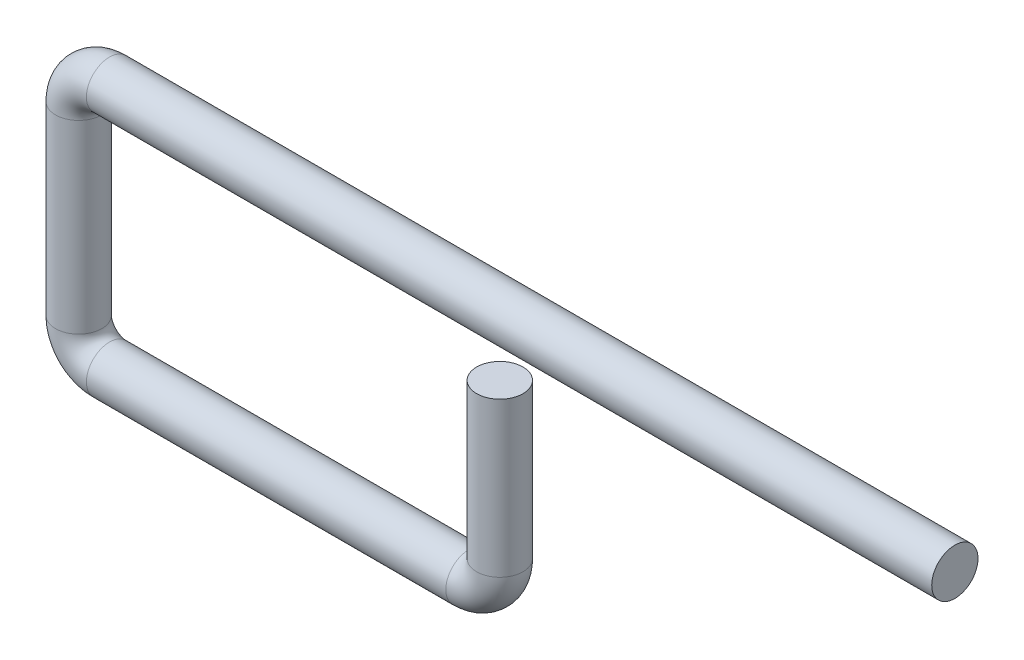
from build123d import *

# Parameters (mm, degrees)
BOLT_ROD_SWEEP_7_5_PROFILE_R = 3.75


with BuildPart() as part:
    # Bolt Rod Sweep Ø7.5: sweep along a path in Bolt Rod Path
    with BuildLine(Plane.XY) as bolt_rod_sweep_7_5_path:
        Line((0, 0), (0, -25))
        ThreePointArc((0, -25), (-1.464466094, -28.535533906), (-5, -30))
        Line((-5, -30), (-63.25, -30))
        ThreePointArc((-63.25, -30), (-66.785533906, -28.535533906), (-68.25, -25))
        Line((-68.25, -25), (-68.25, 5))
        ThreePointArc((-68.25, 5), (-66.785533906, 8.535533906), (-63.25, 10))
        Line((-63.25, 10), (73.75, 10))
    # Bolt Rod Sweep Ø7.5 profile (on start of the path) → Bolt Rod Sweep Ø7.5 (sweep)
    with BuildSketch(Plane(origin=(0, 0, 0), x_dir=(-1, 0, 0), z_dir=(0, -1, 0))):
        Circle(BOLT_ROD_SWEEP_7_5_PROFILE_R)
    sweep(path=bolt_rod_sweep_7_5_path.line)


solid = part.part
